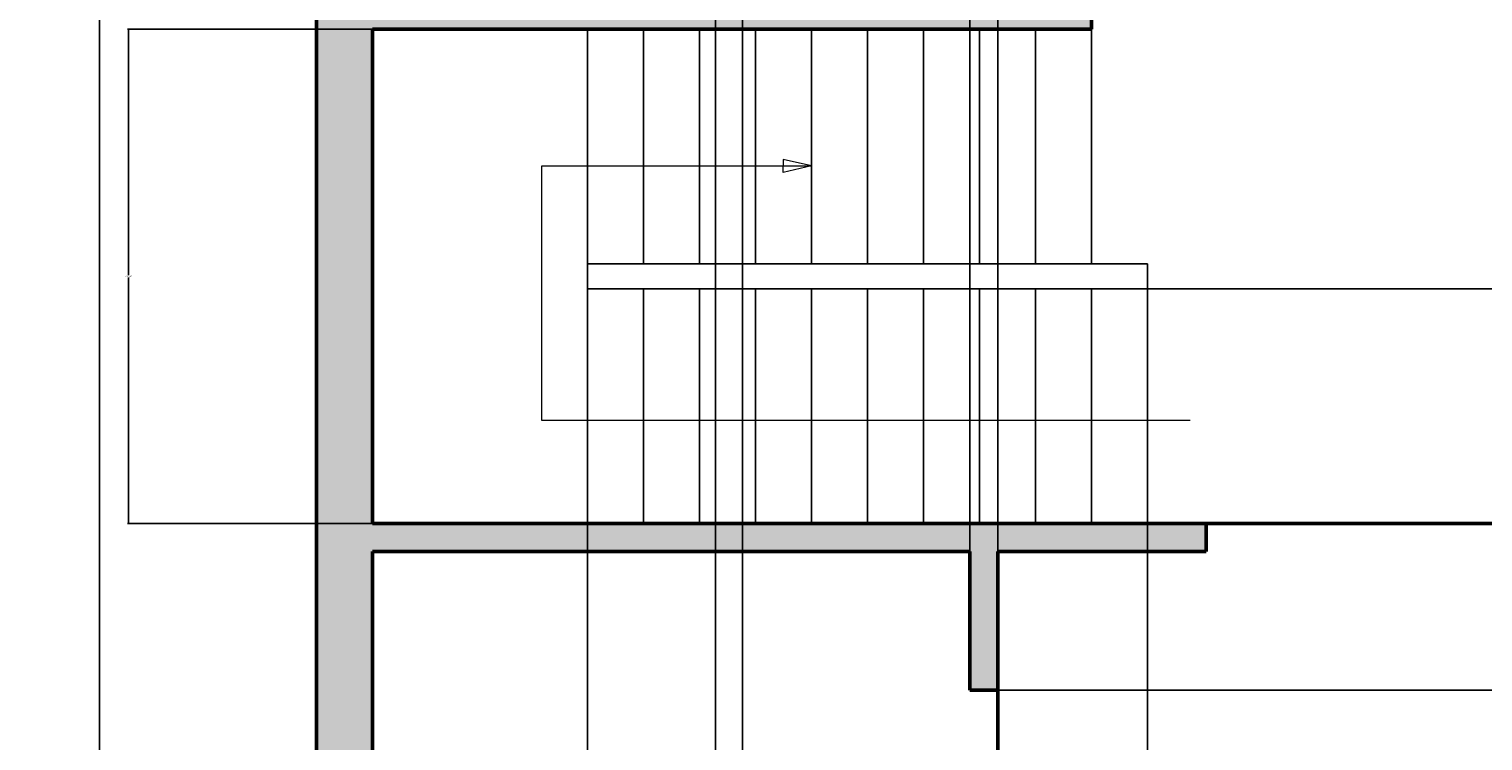
# Model space of a CAD drawing. Units: inches. Extents: x -15 to 420, y -514 to 86.
# Tile 2 of 8: x -15 to 218, y -365 to -251. Entities that reach past the tile are written whole.
import ezdxf

# ---------------------------------------------------------------- set-up
doc = ezdxf.new("R2010")
doc.units = ezdxf.units.IN
doc.header["$MEASUREMENT"] = 0
for name, color, linetype, lineweight in [('A-ANNO-DIMS', 2, 'Continuous', 18), ('A-ANNO-SYMB', 7, 'Continuous', 18), ('A-FLOR-STRS', 7, 'Continuous', 25), ('A-WALL', 7, 'Continuous', 50), ('A-WALL-PATT', 8, 'Continuous', 13)]:
    doc.layers.add(name, color=color, linetype=linetype, lineweight=lineweight)
doc.styles.get("Standard").update_dxf_attribs({"font": 'arial.ttf'})
doc.dimstyles.get("Standard").update_dxf_attribs({"dimtxt": 0.18, "dimasz": 0.18, "dimexe": 0.18, "dimexo": 0.0625, "dimgap": 0.09, "dimtad": 0, "dimtih": 1, "dimtoh": 1, "dimdec": 0, "dimzin": 0, "dimdsep": 46, "dimlunit": 3, "dimtxsty": 'Standard', "dimcen": 0.09, "dimadec": 0, "dimazin": 0, "dimtfac": 1, "dimtdec": 0, "dimtofl": 0, "dimtmove": 0, "dimatfit": 3, "dimfxl": 1, "dimtolj": 1, "dimtzin": 0, "dimarcsym": 0})

# ---------------------------------------------------------------- blocks, each defined once
blk = doc.blocks.new('*D2')
at = {"layer": 'A-ANNO-DIMS', "color": 0, "lineweight": -2, "transparency": 16777216}
for p, q in [((30.86, 13.12), (-4.15, 13.12)), ((-3.97, 12.94), (-3.97, -222.22)), ((-3.97, -463.7), (-3.97, -228.53)), ((30.86, -463.88), (-4.15, -463.88))]:
    blk.add_line(p, q, dxfattribs=at)
at = {"layer": 'A-ANNO-DIMS', "color": 0, "transparency": 16777216}
for points in [[(-4, 12.94), (-3.94, 12.94), (-3.97, 13.12)], [(-4, -463.7), (-3.94, -463.7), (-3.97, -463.88)]]:
    blk.add_solid(points, dxfattribs=at)
at = {"layer": 'Defpoints', "color": 0, "transparency": 16777216}
for p in [(30.92, 13.12), (-3.97, -463.88), (30.92, -463.88)]:
    blk.add_point(p, dxfattribs=at)
at = {"layer": 'A-ANNO-DIMS', "color": 0, "transparency": 16777216, "insert": (-3.97, -225.38), "char_height": 6, "attachment_point": 5}
blk.add_mtext('\\A1;39\'-9"', dxfattribs=at)
blk = doc.blocks.new('*D47')
at = {"layer": 'A-ANNO-DIMS', "color": 0, "lineweight": -2, "transparency": 16777216}
for p, q in [((164.57, -292.63), (419.8, -292.63)), ((419.62, -292.81), (419.62, -311.32)), ((419.62, -330.2), (419.62, -311.69)), ((164.57, -330.38), (419.8, -330.38))]:
    blk.add_line(p, q, dxfattribs=at)
at = {"layer": 'A-ANNO-DIMS', "color": 0, "transparency": 16777216}
for points in [[(419.59, -292.81), (419.65, -292.81), (419.62, -292.63)], [(419.59, -330.2), (419.65, -330.2), (419.62, -330.38)]]:
    blk.add_solid(points, dxfattribs=at)
at = {"layer": 'Defpoints', "color": 0, "transparency": 16777216}
for p in [(164.51, -292.63), (164.51, -330.38), (419.62, -330.38)]:
    blk.add_point(p, dxfattribs=at)
at = {"layer": 'A-ANNO-DIMS', "color": 0, "transparency": 16777216, "insert": (419.62, -311.5), "char_height": 0.18, "attachment_point": 5}
blk.add_mtext('\\A1;3\'-2"', dxfattribs=at)
blk = doc.blocks.new('*D49')
at = {"layer": 'A-ANNO-DIMS', "color": 0, "lineweight": -2, "transparency": 16777216}
for p, q in [((74.51, -330.44), (74.51, -494.26)), ((164.51, -330.44), (164.51, -494.26)), ((74.69, -494.08), (119.18, -494.08)), ((164.33, -494.08), (119.84, -494.08))]:
    blk.add_line(p, q, dxfattribs=at)
at = {"layer": 'A-ANNO-DIMS', "color": 0, "transparency": 16777216}
for points in [[(74.69, -494.05), (74.69, -494.11), (74.51, -494.08)], [(164.33, -494.05), (164.33, -494.11), (164.51, -494.08)]]:
    blk.add_solid(points, dxfattribs=at)
at = {"layer": 'Defpoints', "color": 0, "transparency": 16777216}
for p in [(74.51, -330.38), (164.51, -330.38), (164.51, -494.08)]:
    blk.add_point(p, dxfattribs=at)
at = {"layer": 'A-ANNO-DIMS', "color": 0, "transparency": 16777216, "insert": (119.51, -494.08), "char_height": 0.18, "attachment_point": 5}
blk.add_mtext('\\A1;7\'-6"', dxfattribs=at)
blk = doc.blocks.new('*D50')
at = {"layer": 'A-ANNO-DIMS', "color": 0, "lineweight": -2, "transparency": 16777216}
for p, q in [((39.86, -250.88), (0.54, -250.88)), ((0.72, -251.06), (0.72, -290.45)), ((0.72, -330.2), (0.72, -290.81)), ((39.86, -330.38), (0.54, -330.38))]:
    blk.add_line(p, q, dxfattribs=at)
at = {"layer": 'A-ANNO-DIMS', "color": 0, "transparency": 16777216}
for points in [[(0.69, -251.06), (0.75, -251.06), (0.72, -250.88)], [(0.69, -330.2), (0.75, -330.2), (0.72, -330.38)]]:
    blk.add_solid(points, dxfattribs=at)
at = {"layer": 'Defpoints', "color": 0, "transparency": 16777216}
for p in [(39.92, -250.88), (0.72, -330.38), (39.92, -330.38)]:
    blk.add_point(p, dxfattribs=at)
at = {"layer": 'A-ANNO-DIMS', "color": 0, "transparency": 16777216, "insert": (0.72, -290.63), "char_height": 0.18, "attachment_point": 5}
blk.add_mtext('\\A1;6\'-7 1/2"', dxfattribs=at)
blk = doc.blocks.new('*D51')
at = {"layer": 'A-ANNO-DIMS', "color": 0, "lineweight": -2, "transparency": 16777216}
for p, q in [((135.92, -357.09), (135.92, 43.5)), ((136.1, 43.32), (137.64, 43.32)), ((140.24, 43.32), (138.71, 43.32)), ((140.42, -357.09), (140.42, 43.5))]:
    blk.add_line(p, q, dxfattribs=at)
at = {"layer": 'A-ANNO-DIMS', "color": 0, "transparency": 16777216}
for points in [[(136.1, 43.35), (136.1, 43.29), (135.92, 43.32)], [(140.24, 43.35), (140.24, 43.29), (140.42, 43.32)]]:
    blk.add_solid(points, dxfattribs=at)
at = {"layer": 'Defpoints', "color": 0, "transparency": 16777216}
for p in [(140.42, 43.32), (135.92, -357.15), (140.42, -357.15)]:
    blk.add_point(p, dxfattribs=at)
at = {"layer": 'A-ANNO-DIMS', "color": 0, "transparency": 16777216, "insert": (138.17, 43.32), "char_height": 0.18, "attachment_point": 5}
blk.add_mtext('\\A1;0\'-4 1/2"', dxfattribs=at)
blk = doc.blocks.new('*D52')
at = {"layer": 'A-ANNO-DIMS', "color": 0, "lineweight": -2, "transparency": 16777216}
for p, q in [((140.49, -357.15), (419.8, -357.15)), ((419.62, -357.33), (419.62, -375.83)), ((419.62, -394.7), (419.62, -376.2)), ((140.49, -394.88), (419.8, -394.88))]:
    blk.add_line(p, q, dxfattribs=at)
at = {"layer": 'A-ANNO-DIMS', "color": 0, "transparency": 16777216}
for points in [[(419.59, -357.33), (419.65, -357.33), (419.62, -357.15)], [(419.59, -394.7), (419.65, -394.7), (419.62, -394.88)]]:
    blk.add_solid(points, dxfattribs=at)
at = {"layer": 'Defpoints', "color": 0, "transparency": 16777216}
for p in [(140.42, -357.15), (140.42, -394.88), (419.62, -394.88)]:
    blk.add_point(p, dxfattribs=at)
at = {"layer": 'A-ANNO-DIMS', "color": 0, "transparency": 16777216, "insert": (419.62, -376.01), "char_height": 0.18, "attachment_point": 5}
blk.add_mtext('\\A1;3\'-1 1/2"', dxfattribs=at)
blk = doc.blocks.new('*D58')
at = {"layer": 'A-ANNO-DIMS', "color": 0, "lineweight": -2, "transparency": 16777216}
for p, q in [((95.06, -434.9), (95.06, 43.5)), ((95.24, 43.32), (96.7, 43.32)), ((99.24, 43.32), (97.78, 43.32)), ((99.42, -434.9), (99.42, 43.5))]:
    blk.add_line(p, q, dxfattribs=at)
at = {"layer": 'A-ANNO-DIMS', "color": 0, "transparency": 16777216}
for points in [[(95.24, 43.35), (95.24, 43.29), (95.06, 43.32)], [(99.24, 43.35), (99.24, 43.29), (99.42, 43.32)]]:
    blk.add_solid(points, dxfattribs=at)
at = {"layer": 'Defpoints', "color": 0, "transparency": 16777216}
for p in [(99.42, 43.32), (95.06, -434.96), (99.42, -434.96)]:
    blk.add_point(p, dxfattribs=at)
at = {"layer": 'A-ANNO-DIMS', "color": 0, "transparency": 16777216, "insert": (97.24, 43.32), "char_height": 0.18, "attachment_point": 5}
blk.add_mtext('\\A1;0\'-4 1/2"', dxfattribs=at)

msp = doc.modelspace()

# ---------------------------------------------------------------- hatches: boundary and pattern name
at = {"layer": 'A-WALL-PATT'}
h = msp.add_hatch(color=256, dxfattribs=at)
h.dxf.hatch_style = 1
h.paths.add_polyline_path([(266.67, -454.88), (240.92, -454.88), (240.92, -330.38), (236.42, -330.38), (236.42, -454.88), (218.42, -454.88), (218.42, -463.88), (266.67, -463.88)])
h.paths.add_polyline_path([(158.42, -454.88), (140.42, -454.88), (140.42, -394.88), (135.92, -394.88), (135.92, -454.88), (39.92, -454.88), (39.92, -412.88), (30.92, -412.88), (30.92, -463.88), (158.42, -463.88)])
h.paths.add_polyline_path([(39.92, -334.88), (135.92, -334.88), (135.92, -357.15), (140.42, -357.15), (140.42, -334.88), (173.95, -334.88), (173.95, -330.38), (39.92, -330.38), (39.92, -250.88), (155.51, -250.88), (155.51, -246.38), (140.42, -246.38), (140.42, -205.38), (138.17, -205.38), (135.92, -205.38), (135.92, -246.38), (39.92, -246.38), (39.92, -222.38), (30.92, -222.38), (30.92, -376.88), (39.92, -376.88)])
h.paths.add_polyline_path([(389.42, -382.88), (380.42, -382.88), (380.42, -454.88), (380.42, -463.88), (389.42, -463.88)])
h.paths.add_polyline_path([(352.42, -459.38), (352.42, -454.88), (326.67, -454.88), (326.67, -463.88), (352.42, -463.88)])
h.paths.add_polyline_path([(176.92, -169.88), (39.92, -169.88), (39.92, -112.88), (30.92, -112.88), (30.92, -198.38), (39.92, -198.38), (39.92, -174.38), (135.92, -174.38), (135.92, -177.38), (140.42, -177.38), (140.42, -174.38), (176.92, -174.38), (176.92, -172.13)])
h.paths.add_polyline_path([(39.92, 4.12), (93.92, 4.12), (93.92, 13.12), (30.92, 13.12), (30.92, -52.88), (39.92, -52.88)])
h.paths.add_polyline_path([(266.42, 13.12), (153.92, 13.12), (153.92, 4.12), (207.92, 4.12), (207.92, -169.88), (204.92, -169.88), (204.92, -174.38), (215.42, -174.38), (215.42, -169.88), (212.42, -169.88), (212.42, 4.12), (266.42, 4.12)])
h.paths.add_polyline_path([(389.42, 13.12), (326.42, 13.12), (326.42, 4.12), (380.42, 4.12), (380.42, -52.88), (389.42, -52.88)])
h.paths.add_polyline_path([(389.42, -112.88), (380.42, -112.88), (380.42, -169.88), (377.42, -169.88), (377.42, -174.38), (380.42, -174.38), (380.42, -198.38), (389.42, -198.38)])
h.paths.add_polyline_path([(349.42, -172.13), (349.42, -169.88), (243.42, -169.88), (243.42, -172.13), (243.42, -174.38), (279.92, -174.38), (279.92, -250.88), (380.42, -250.88), (380.42, -322.88), (389.42, -322.88), (389.42, -222.38), (380.42, -222.38), (380.42, -246.38), (284.42, -246.38), (284.42, -174.38), (349.42, -174.38)])

# ---------------------------------------------------------------- linework, layer by layer
at = {"layer": 'A-ANNO-SYMB'}
for p, q in [((67.14, -313.79), (67.14, -272.89)), ((67.14, -272.89), (110.51, -272.89)), ((110.51, -272.89), (105.94, -271.84)), ((105.94, -271.84), (105.94, -272.89)), ((110.51, -272.89), (105.94, -273.94)), ((105.94, -273.94), (105.94, -272.89)), ((171.35, -313.79), (67.14, -313.79))]:
    msp.add_line(p, q, dxfattribs=at)
at = {"layer": 'A-FLOR-STRS'}
for p, q in [((74.51, -250.88), (74.51, -330.38)), ((83.51, -250.88), (83.51, -288.63)), ((92.51, -250.88), (92.51, -288.63)), ((101.51, -250.88), (101.51, -288.63)), ((110.51, -250.88), (110.51, -288.63)), ((119.51, -250.88), (119.51, -288.63)), ((128.51, -250.88), (128.51, -288.63)), ((137.51, -250.88), (137.51, -288.63)), ((146.51, -250.88), (146.51, -288.63)), ((155.51, -250.88), (155.51, -288.63)), ((74.51, -288.63), (164.51, -288.63)), ((164.51, -288.63), (164.51, -330.38)), ((74.51, -292.63), (164.51, -292.63)), ((83.51, -292.63), (83.51, -330.38)), ((92.51, -292.63), (92.51, -330.38)), ((101.51, -292.63), (101.51, -330.38)), ((110.51, -292.63), (110.51, -330.38)), ((119.51, -292.63), (119.51, -330.38)), ((128.51, -292.63), (128.51, -330.38)), ((137.51, -292.63), (137.51, -330.38)), ((146.51, -292.63), (146.51, -330.38)), ((155.51, -292.63), (155.51, -330.38))]:
    msp.add_line(p, q, dxfattribs=at)
at = {"layer": 'A-WALL'}
for p, q in [((30.92, 13.12), (30.92, -463.88)), ((155.51, -246.38), (155.51, -250.88)), ((39.92, -250.88), (155.51, -250.88)), ((39.92, -250.88), (39.92, -330.38)), ((39.92, -330.38), (240.92, -330.38)), ((173.95, -330.38), (173.95, -334.88)), ((39.92, -334.88), (135.92, -334.88)), ((39.92, -334.88), (39.92, -454.88)), ((135.92, -334.88), (135.92, -357.15)), ((140.42, -334.88), (140.42, -454.88)), ((140.42, -334.88), (173.95, -334.88)), ((140.42, -357.15), (135.92, -357.15))]:
    msp.add_line(p, q, dxfattribs=at)

# ---------------------------------------------------------------- dimensions: what is measured, and where the dimension line sits
at = {"layer": 'A-ANNO-DIMS'}
for base, p1, p2, picture, middle in [((99.42, 43.32), (95.06, -434.96), (99.42, -434.96), '*D58', (97.24, 43.32)), ((140.42, 43.32), (135.92, -357.15), (140.42, -357.15), '*D51', (138.17, 43.32)), ((164.51, -494.08), (74.51, -330.38), (164.51, -330.38), '*D49', (119.51, -494.08))]:
    dim = msp.add_linear_dim(base=base, p1=p1, p2=p2, dimstyle='Standard', override={"dimdec": 1, "dimlfac": 1, "dimrnd": 0, "dimzin": 1, "dimdsep": 46, "dimlunit": 4, "dimfrac": 2}, dxfattribs=at)
    dim.commit()
    dim.dimension.update_dxf_attribs({"geometry": picture, "text_midpoint": middle})
for base, p1, p2, override, picture, middle in [((-3.97, -463.88), (30.92, 13.12), (30.92, -463.88), {"dimtxt": 6, "dimclrd": 0, "dimclre": 0, "dimclrt": 0}, '*D2', (-3.97, -225.38)), ((0.72, -330.38), (39.92, -250.88), (39.92, -330.38), {"dimdec": 1, "dimlfac": 1, "dimrnd": 0, "dimzin": 1, "dimdsep": 46, "dimlunit": 4, "dimfrac": 2}, '*D50', (0.72, -290.63)), ((419.624858, -330.379493), (164.510771, -292.629493), (164.510771, -330.379493), {"dimdec": 1, "dimlfac": 1, "dimrnd": 0, "dimzin": 1, "dimdsep": 46, "dimlunit": 4, "dimfrac": 2}, '*D47', (419.624858, -311.504493)), ((419.62, -394.88), (140.42, -357.15), (140.42, -394.88), {"dimdec": 1, "dimlfac": 1, "dimrnd": 0, "dimzin": 1, "dimdsep": 46, "dimlunit": 4, "dimfrac": 2}, '*D52', (419.62, -376.01))]:
    dim = msp.add_linear_dim(base=base, p1=p1, p2=p2, angle=90, dimstyle='Standard', override=override, dxfattribs=at)
    dim.commit()
    dim.dimension.update_dxf_attribs({"geometry": picture, "text_midpoint": middle})

doc.saveas('drawing.dxf')
